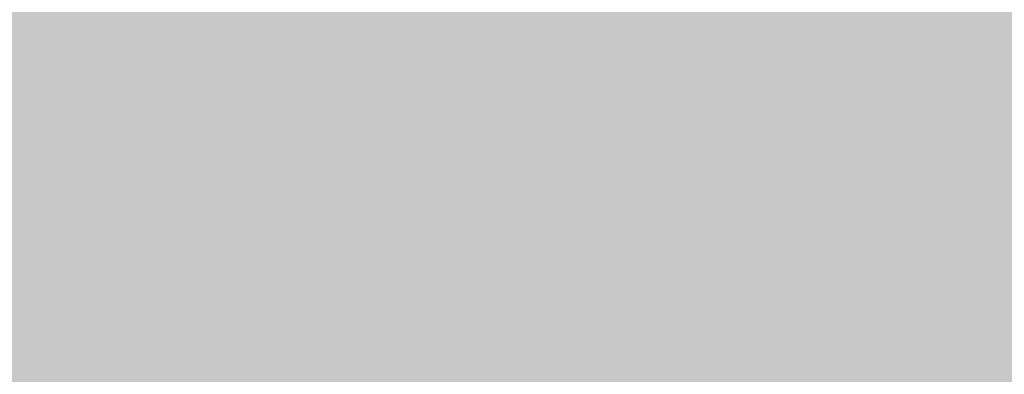
# Model space of a CAD drawing. Units: feet. Extents: x 3168 to 4724, y 827 to 1477.
# Tile 174 of 256: x 3303.032 to 3307.378, y 1096.781 to 1098.344. Entities that reach past the tile are written whole.
import ezdxf

# ---------------------------------------------------------------- set-up
doc = ezdxf.new("R2010")
doc.units = ezdxf.units.FT
doc.layers.add('A-ELEV-PATT', color=8, linetype='Continuous', lineweight=13)

msp = doc.modelspace()

# ---------------------------------------------------------------- hatches: boundary and pattern name
at = {"layer": 'A-ELEV-PATT'}
h = msp.add_hatch(color=256, dxfattribs=at)
h.dxf.hatch_style = 1
edge = h.paths.add_edge_path()
edge.add_ellipse((3552.9058, 979.2201), major_axis=(36.7449, 0), ratio=0.4848485, start_angle=0, end_angle=360)
edge = h.paths.add_edge_path()
edge.add_ellipse((3559.8916, 929.2523), major_axis=(36.7449, 0), ratio=0.4848485, start_angle=0, end_angle=360)
edge = h.paths.add_edge_path()
edge.add_line((3299.3168, 1198.6061), (3479.9167, 1198.6061))
edge.add_line((3479.9167, 1198.6061), (3479.9167, 1209.8686))
edge.add_spline(control_points=[(3479.9167, 1209.8686), (3464.3012, 1209.8686), (3448.6856, 1209.8686), (3410.9491, 1209.8686), (3388.8282, 1209.8686), (3355.6469, 1209.8686), (3344.5864, 1209.8686), (3327.9957, 1209.8686), (3322.4655, 1209.8686), (3314.1702, 1209.8686), (3311.4051, 1209.8686), (3307.2574, 1209.8686), (3305.8748, 1209.8686), (3303.801, 1209.8686), (3303.1097, 1209.8686), (3302.0728, 1209.8686), (3301.7272, 1209.8686), (3301.2087, 1209.8686), (3301.0359, 1209.8686), (3300.7767, 1209.8686), (3300.6903, 1209.8686), (3300.5606, 1209.8686), (3300.5174, 1209.8686), (3300.4526, 1209.8686), (3300.431, 1209.8686), (3300.3986, 1209.8686), (3300.3878, 1209.8686), (3300.3662, 1209.8686), (3300.3457, 1209.8686), (3300.3455, 1209.8686), (3300.3455, 1209.8686), (3300.3433, 1209.8686), (3300.3411, 1209.8686), (3300.3379, 1209.8686), (3300.3368, 1209.8686), (3300.3339, 1209.8686), (3300.3321, 1209.8686), (3300.3255, 1209.8686), (3300.3207, 1209.8686), (3300.3109, 1209.8686), (3300.306, 1209.8686), (3300.2905, 1209.8686), (3300.28, 1209.8686), (3300.2324, 1209.8688), (3300.1953, 1209.869), (3299.9511, 1209.8706), (3299.7448, 1209.8743), (3299.4368, 1209.8833), (3299.3344, 1209.8868), (3299.1811, 1209.8929), (3299.13, 1209.8951), (3298.6522, 1209.9168), (3298.2295, 1209.9457), (3297.6016, 1210.0024), (3297.3934, 1210.0235), (3297.0827, 1210.0583), (3296.9793, 1210.0705), (3296.293, 1210.1549), (3295.7181, 1210.2434), (3294.8687, 1210.3989), (3294.5877, 1210.4545), (3294.1693, 1210.5433), (3294.0304, 1210.5739), (3291.7071, 1211.1012), (3289.6536, 1211.8134), (3285.7763, 1213.564), (3283.9514, 1214.6035), (3280.5122, 1216.9801), (3278.8972, 1218.3176), (3276.3799, 1220.8295), (3275.416, 1221.9177), (3274.0393, 1223.7077), (3273.581, 1224.3495), (3273.1432, 1225.0163)], knot_values=[39.119033, 39.119033, 39.119033, 39.119033, 39.286353, 39.286353, 39.523379, 39.523379, 39.641892, 39.641892, 39.701148, 39.701148, 39.730777, 39.730777, 39.745591, 39.745591, 39.752998, 39.752998, 39.756701, 39.756701, 39.758553, 39.758553, 39.759479, 39.759479, 39.759942, 39.759942, 39.760173, 39.760173, 39.760289, 39.760289, 39.760405, 39.760405, 39.760463, 39.760463, 39.763389, 39.763389, 39.764851, 39.764851, 39.767304, 39.767304, 39.773825, 39.773825, 39.78057, 39.78057, 39.79477, 39.79477, 39.845194, 39.845194, 40.126715, 40.126715, 40.267476, 40.267476, 40.337856, 40.337856, 40.927023, 40.927023, 41.221606, 41.221606, 41.368898, 41.368898, 42.202622, 42.202622, 42.619485, 42.619485, 42.827916, 42.827916, 46.118323, 46.118323, 49.408731, 49.408731, 52.699139, 52.699139, 54.927489, 54.927489, 56.104228, 56.104228, 56.104228, 56.104228], weights=[1, 1, 1, 1, 1, 1, 1, 1, 1, 1, 1, 1, 1, 1, 1, 1, 1, 1, 1, 1, 1, 1, 1, 1, 1, 1, 1, 1, 1, 1, 1, 1, 1, 1, 1, 1, 1, 1, 1, 1, 1, 1, 1, 1, 1, 1, 1, 1, 1, 1, 1, 1, 1, 1, 1, 1, 1, 1, 1, 1, 1, 1, 1, 1, 1, 1, 1, 1, 1, 1, 1, 1, 1, 1], degree=3, periodic=0)
edge.add_line((3273.1432, 1225.0163), (3273.1432, 1099.0163))
edge.add_line((3273.1432, 1099.0163), (3299.3168, 1099.0163))
edge.add_line((3299.3168, 1099.0163), (3299.3168, 1198.6061))
edge = h.paths.add_edge_path()
edge.add_line((3304.7584, 1324.1581), (3479.9167, 1324.1581))
edge.add_line((3479.9167, 1324.1581), (3479.9167, 1335.7146))
edge.add_line((3479.9167, 1335.7146), (3269.1616, 1335.7146))
edge.add_spline(control_points=[(3269.1616, 1335.7146), (3264.0242, 1335.7146), (3258.3641, 1328.9582), (3259.2643, 1323.9003)], knot_values=[0, 0, 0, 0, 15.412191, 15.412191, 15.412191, 15.412191], degree=3, periodic=0)
edge.add_line((3259.2643, 1323.9003), (3265.5168, 1288.7691))
edge.add_line((3265.5168, 1288.7691), (3275.2651, 1261.5456))
edge.add_line((3275.2651, 1261.5456), (3304.7584, 1261.5456))
edge.add_line((3304.7584, 1261.5456), (3304.7584, 1324.1581))
h = msp.add_hatch(color=256, dxfattribs=at)
h.dxf.hatch_style = 1
h.paths.add_polyline_path([(3384.5252, 1099.0163), (3335.0292, 1099.0163), (3299.3168, 1099.0163), (3273.1432, 1099.0163), (3217.5654, 1099.0163), (3168.0693, 827.1163), (3335.0292, 827.1163)])

doc.saveas('drawing.dxf')
